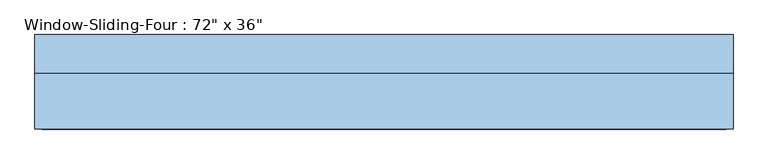
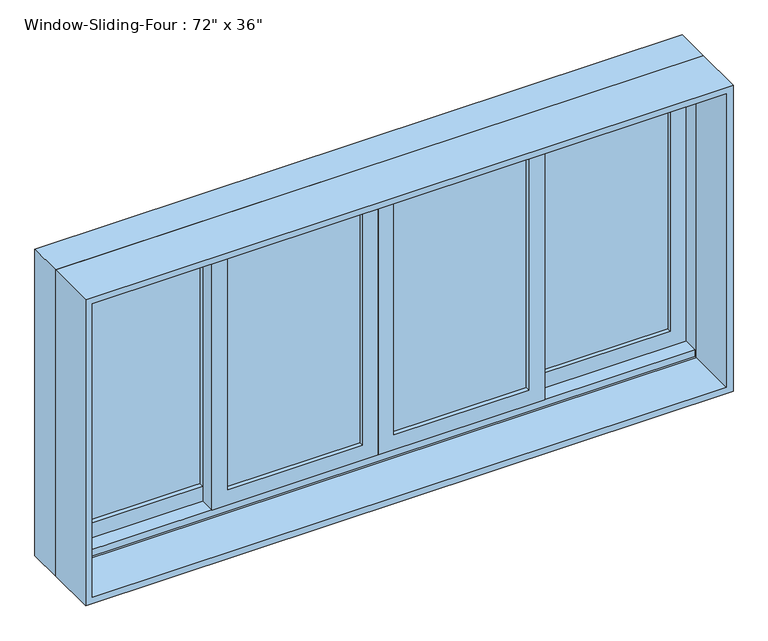
"""IFC4 building model written with IfcOpenShell, lengths in millimetres: window geometry."""

from ifc_helpers import new_model, si_unit, frame, origin, place, context, project, spatial, polyline, outline, extrude, faceted_brep, source, transform, mapped, element, save


def window_58cce754(model_context):
    return source(origin(), model_context, "Body", "SolidModel", [
        extrude(outline(polyline([(933.45, -895.35), (933.45, -425.45), (1809.75, -425.45), (1809.75, -895.35), (933.45, -895.35)]), holes=[polyline([(1765.3, -469.9), (996.95, -469.9), (996.95, -850.9), (1765.3, -850.9), (1765.3, -469.9)])]), frame((0.0, 78.74, 0.0), z_axis=(0.0, 1.0, 0.0), x_axis=(0.0, 0.0, 1.0)), (0.0, 0.0, 1.0), 44.45),
        extrude(outline(polyline([(-469.9, 110.49), (-469.9, 104.14), (-850.9, 104.14), (-850.9, 110.49), (-469.9, 110.49)])), frame((0.0, 0.0, 996.95), z_axis=(0.0, 0.0, 1.0), x_axis=(1.0, 0.0, 0.0)), (0.0, 0.0, 1.0), 768.35),
        extrude(outline(polyline([(-469.9, 97.79), (-469.9, 91.44), (-850.9, 91.44), (-850.9, 97.79), (-469.9, 97.79)])), frame((0.0, 0.0, 996.95), z_axis=(0.0, 0.0, 1.0), x_axis=(1.0, 0.0, 0.0)), (0.0, 0.0, 1.0), 768.35),
        extrude(outline(polyline([(-44.45, 66.04), (-44.45, 59.69), (-425.45, 59.69), (-425.45, 66.04), (-44.45, 66.04)])), frame((0.0, 0.0, 996.95), z_axis=(0.0, 0.0, 1.0), x_axis=(1.0, 0.0, 0.0)), (0.0, 0.0, 1.0), 768.35),
        extrude(outline(polyline([(-44.45, 53.34), (-44.45, 46.99), (-425.45, 46.99), (-425.45, 53.34), (-44.45, 53.34)])), frame((0.0, 0.0, 996.95), z_axis=(0.0, 0.0, 1.0), x_axis=(1.0, 0.0, 0.0)), (0.0, 0.0, 1.0), 768.35),
        extrude(outline(polyline([(1828.8, -914.4), (914.4, -914.4), (914.4, 914.4), (1828.8, 914.4), (1828.8, -914.4)]), holes=[polyline([(1809.75, 895.35), (933.45, 895.35), (933.45, -895.35), (1809.75, -895.35), (1809.75, 895.35)])]), frame((0.0, -118.11, 0.0), z_axis=(0.0, 1.0, 0.0), x_axis=(0.0, 0.0, 1.0)), (0.0, 0.0, 1.0), 146.05),
        extrude(outline(polyline([(952.5, 469.9), (1809.75, 469.9), (1809.75, 0.0), (952.5, 0.0), (952.5, 469.9)]), holes=[polyline([(996.95, 44.45), (1765.3, 44.45), (1765.3, 425.45), (996.95, 425.45), (996.95, 44.45)])]), frame((0.0, 34.29, 0.0), z_axis=(0.0, 1.0, 0.0), x_axis=(0.0, 0.0, 1.0)), (0.0, 0.0, 1.0), 44.45),
        extrude(outline(polyline([(1809.75, -469.9), (952.5, -469.9), (952.5, 0.0), (1809.75, 0.0), (1809.75, -469.9)]), holes=[polyline([(1765.3, -44.45), (996.95, -44.45), (996.95, -425.45), (1765.3, -425.45), (1765.3, -44.45)])]), frame((0.0, 34.29, 0.0), z_axis=(0.0, 1.0, 0.0), x_axis=(0.0, 0.0, 1.0)), (0.0, 0.0, 1.0), 44.45),
        extrude(outline(polyline([(425.45, 66.04), (425.45, 59.69), (44.45, 59.69), (44.45, 66.04), (425.45, 66.04)])), frame((0.0, 0.0, 996.95), z_axis=(0.0, 0.0, 1.0), x_axis=(1.0, 0.0, 0.0)), (0.0, 0.0, 1.0), 768.35),
        extrude(outline(polyline([(425.45, 53.34), (425.45, 46.99), (44.45, 46.99), (44.45, 53.34), (425.45, 53.34)])), frame((0.0, 0.0, 996.95), z_axis=(0.0, 0.0, 1.0), x_axis=(1.0, 0.0, 0.0)), (0.0, 0.0, 1.0), 768.35),
        extrude(outline(polyline([(850.9, 110.49), (850.9, 104.14), (469.9, 104.14), (469.9, 110.49), (850.9, 110.49)])), frame((0.0, 0.0, 996.95), z_axis=(0.0, 0.0, 1.0), x_axis=(1.0, 0.0, 0.0)), (0.0, 0.0, 1.0), 768.35),
        extrude(outline(polyline([(850.9, 97.4725303), (850.9, 91.44), (469.9, 91.44), (469.9, 97.4725303), (850.9, 97.4725303)])), frame((0.0, 0.0, 996.95), z_axis=(0.0, 0.0, 1.0), x_axis=(1.0, 0.0, 0.0)), (0.0, 0.0, 1.0), 768.35),
        extrude(outline(polyline([(933.45, 895.35), (1809.75, 895.35), (1809.75, 425.45), (933.45, 425.45), (933.45, 895.35)]), holes=[polyline([(1765.3, 469.9), (1765.3, 850.9), (996.95, 850.9), (996.95, 469.9), (1765.3, 469.9)])]), frame((0.0, 78.74, 0.0), z_axis=(0.0, 1.0, 0.0), x_axis=(0.0, 0.0, 1.0)), (0.0, 0.0, 1.0), 44.45),
        faceted_brep([(-914.4, 27.94, 914.4), (-914.4, 129.54, 914.4), (914.4, 129.54, 914.4), (914.4, 27.94, 914.4), (-873.4778905, 129.54, 1787.8778905), (-873.4778905, 123.19, 1787.8778905), (-873.4778905, 123.19, 933.45), (-873.4778905, 129.54, 933.45), (873.4778905, 123.19, 1787.8778905), (873.4778905, 123.19, 933.45), (895.35, 123.19, 933.45), (895.35, 123.19, 1809.75), (-895.35, 123.19, 1809.75), (-895.35, 123.19, 933.45), (-895.35, 27.94, 1809.75), (-895.35, 27.94, 933.45), (-895.35, 34.29, 933.45), (-895.35, 34.29, 952.5), (-895.35, 78.74, 952.5), (-895.35, 78.74, 933.45), (914.4, 27.94, 1828.8), (-914.4, 27.94, 1828.8), (895.35, 27.94, 1809.75), (895.35, 27.94, 933.45), (-914.4, 129.54, 1828.8), (914.4, 129.54, 1828.8), (873.4778905, 129.54, 933.45), (873.4778905, 129.54, 1787.8778905), (895.35, 78.74, 933.45), (895.35, 78.74, 952.5), (895.35, 34.29, 952.5), (895.35, 34.29, 933.45)], [[[0, 1, 2, 3]], [[4, 5, 6, 7]], [[5, 8, 9, 10, 11, 12, 13, 6]], [[12, 14, 15, 16, 17, 18, 19, 13]], [[0, 3, 20, 21], [22, 23, 15, 14]], [[24, 1, 0, 21]], [[2, 1, 24, 25], [4, 7, 26, 27]], [[5, 4, 27, 8]], [[12, 11, 22, 14]], [[21, 20, 25, 24]], [[8, 27, 26, 9]], [[22, 11, 10, 28, 29, 30, 31, 23]], [[20, 3, 2, 25]], [[26, 7, 6, 13, 19, 28, 10, 9]], [[28, 19, 18, 29]], [[29, 18, 17, 30]], [[30, 17, 16, 31]], [[15, 23, 31, 16]]]),
    ])


if __name__ == "__main__":
    model = new_model("IFC4")
    model_context = context("Model", 3, world=origin())
    ifc_project = project(units=[si_unit("LENGTHUNIT", "METRE", prefix="MILLI")], contexts=[model_context])
    site = spatial("IfcSite", under=ifc_project)
    building = spatial("IfcBuilding", under=site)
    placement = place(None, origin())
    window_shape = window_58cce754(model_context)
    element("IfcWindow", 1, ObjectType="Window-Sliding-Four : 72\" x 36\"", at=placement, inside=building, context=model_context, shape_type="MappedRepresentation", body=[
        mapped(window_shape, transform((0.0, 0.0, 0.0), x_axis=(1.0, 0.0, 0.0), y_axis=(0.0, 1.0, 0.0), z_axis=(0.0, 0.0, 1.0))),
    ])
    save(model, "model.ifc")

# Revit data of these elements
# Type "Window-Sliding-Four : 72\" x 36\""
#   Type Mark = "20"
#   Fire Rating = "0.5h"
#   Assembly Code = "B2020100"
#   Analytic Construction = "Double glazing - domestic"
#   Window Inset [instance default] = 0' - 0"
#   Wall Thickness [instance default] = 0' - 6"
#   Visual Light Transmittance = 0.81
#   Thermal Resistance (R) = 1.8146 (h·ft²·°F)/BTU
#   Solar Heat Gain Coefficient = 0.76
#   Interior Wall Closure [instance default] = 0' - 2 19/32"
#   Heat Transfer Coefficient (U) = 0.5511 BTU/(h·ft²·°F)
#   Frame Extension [instance default] = 0' - 0 1/4"
#   Exterior Wall Closure [instance default] = 0' - 1 1/4"
#   Rough Width = 6' - 0 1/2"
#   Rough Height = 3' - 0 1/2"
#   Height = 3' - 0"
#   Extension Jamb [instance default] = 0' - 2 3/4"
#   Default Sill Height = 3' - 0"
#   Width = 6' - 0"
#   Middle Muntin Visibility = yes
#   Interior Trim Visibility [instance default] = yes
#   Indicator Visibility [instance default] = yes
#   Exterior Trim Visibility [instance default] = yes
#   Side Muntin Visibility = yes
#   Extension Jamb Visibility [instance default] = yes
#   Interior Trim Material = Wood - Stained
#   Muntin Pattern = Muntin Pattern_2x2 : Muntin Pattern_2x2
#   Interior Trim = Trim-Window-Interior-Flat : Picture Frame
#   Interior Frame Material = Wood - Stained
#   Glass Panel Material = Glass
#   Exterior Trim Material = Clad - White
#   Exterior Trim = Trim-Window-Exterior-Flat : with Sill
#   Exterior Frame Material = Clad - White
#   Wall Closure = (empty or 0)
# Element 1 (IfcWindow, "Window-Sliding-Four : 72\" x 36\"")
#   Wall Thickness = 0' - 9"
#   Interior Wall Closure = 0' - 2 3/4"
#   Extension Jamb = 0' - 5 3/4"
#   Materials on its faces: "Wood - Stained", "Glass", "Clad - White"
# Materials
#   "Wood - Stained": class "Wood", colour RGB 224 178 126, transparency 0, Cost = 0
#   "Glass": class "Glass", colour RGB 0 128 192, transparency 0.75, Description = "Soda Lime Glass", Cost = 0
#   "Clad - White": class "Wood", colour RGB 242 242 238, transparency 0, Cost = 0
